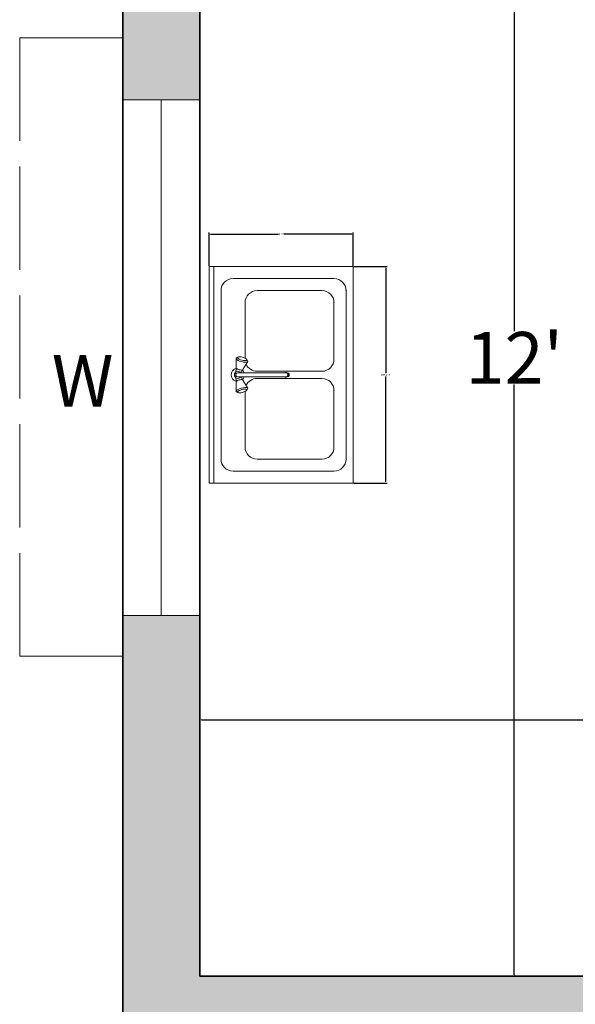
# Model space of a CAD drawing. Units: inches. Extents: x -5 to 482, y -460 to 66.
# Tile 17 of 31: x 21 to 86, y -143 to -29. Entities that reach past the tile are written whole.
import ezdxf

# ---------------------------------------------------------------- set-up
doc = ezdxf.new("R2010")
doc.units = ezdxf.units.IN
doc.header["$MEASUREMENT"] = 0
doc.linetypes.add('ACAD_ISO02W100', pattern=[15, 12, -3])
for name, color, linetype, lineweight in [('A-ANNO-DIMS', 2, 'Continuous', 18), ('A-ANNO-TEXT', 7, 'Continuous', 18), ('A-FLOR-FIXT', 9, 'Continuous', 18), ('A-GLAZ', 4, 'Continuous', 18), ('A-GLAZ-OVHD', 4, 'ACAD_ISO02W100', 13), ('A-WALL', 7, 'Continuous', 35), ('A-WALL-PATT', 152, 'Continuous', 13)]:
    doc.layers.add(name, color=color, linetype=linetype, lineweight=lineweight)
doc.styles.get("Standard").update_dxf_attribs({"font": 'arial.ttf'})
doc.dimstyles.get("Standard").update_dxf_attribs({"dimtxt": 0.18, "dimasz": 0.18, "dimexe": 0.18, "dimexo": 0.0625, "dimgap": 0.09, "dimtad": 0, "dimtih": 1, "dimtoh": 1, "dimdec": 0, "dimzin": 0, "dimdsep": 46, "dimlunit": 3, "dimtxsty": 'Standard', "dimcen": 0.09, "dimadec": 0, "dimazin": 0, "dimtfac": 1, "dimtdec": 0, "dimtofl": 0, "dimtmove": 0, "dimatfit": 3, "dimfxl": 1, "dimtolj": 1, "dimtzin": 0, "dimarcsym": 0})

# ---------------------------------------------------------------- blocks, each defined once
blk = doc.blocks.new('М07 600х900')
for p, q in [((0, 600), (-900, 600)), ((-900, 0), (-900, 600)), ((-900, 0), (-900, 600)), ((0, 580), (-900, 580)), ((0, 0), (0, 600)), ((0, 0), (0, 600)), ((-800, 550), (-100, 550)), ((-850, 80), (-850, 500)), ((-476.6, 488.7), (-472.7, 496.5)), ((-472.7, 496.5), (-466.5, 502.7)), ((-466.5, 502.7), (-458.7, 506.6)), ((-462.1, 488.8), (-454.6, 494.3)), ((-458.7, 506.6), (-450, 508)), ((-454.6, 494.3), (-445.4, 494.3)), ((-450, 508), (-441.3, 506.6)), ((-445.4, 494.3), (-437.9, 488.8)), ((-441.3, 506.6), (-433.5, 502.7)), ((-433.5, 502.7), (-427.3, 496.5)), ((-427.3, 496.5), (-423.4, 488.7)), ((-50, 500), (-50, 80)), ((-524.9, 472.1), (-524.8, 476.7)), ((-524.3, 466.5), (-524.9, 472.1)), ((-524.8, 476.7), (-523.8, 479.9)), ((-523, 460.4), (-524.3, 466.5)), ((-520.9, 485.6), (-523.8, 479.9)), ((-523.8, 479.9), (-522.2, 481.3)), ((-521.1, 454.5), (-523, 460.4)), ((-522.2, 481.3), (-520.1, 480.9)), ((-518.8, 449.4), (-521.1, 454.5)), ((-520.9, 485.6), (-518.9, 487.4)), ((-520.1, 480.9), (-517.7, 478.6)), ((-479.6, 487.6), (-518.9, 487.4)), ((-518.9, 487.4), (-516.3, 486.8)), ((-517.7, 478.6), (-515.3, 474.7)), ((-516.3, 486.8), (-513.3, 484)), ((-515.3, 474.7), (-513, 469.5)), ((-513.3, 484), (-510.2, 479.1)), ((-513, 469.5), (-511.1, 463.6)), ((-511.1, 463.6), (-509.8, 457.6)), ((-510.2, 479.1), (-507.4, 472.6)), ((-509.8, 457.6), (-509.2, 452)), ((-509.2, 452), (-509.4, 447.3)), ((-507.4, 472.6), (-505, 465.3)), ((-471.8, 458.6), (-506, 439.1)), ((-505, 465.3), (-503.4, 457.7)), ((-503.4, 457.7), (-502.6, 450.7)), ((-502.6, 450.7), (-502.8, 444.9)), ((-479.6, 487.6), (-478, 487.3)), ((-478, 487.3), (-476.2, 485.5)), ((-477, 486.3), (-476.6, 488.7)), ((-461.4, 489.4), (-476.2, 485.4)), ((-476.2, 485.5), (-474.4, 482.6)), ((-474.4, 482.6), (-472.7, 478.7)), ((-472.7, 478.7), (-471.2, 474.3)), ((-470.6, 459.7), (-471.8, 458.6)), ((-471.2, 474.3), (-470.3, 469.8)), ((-469.9, 462.1), (-470.6, 459.7)), ((-470.3, 469.8), (-469.8, 465.6)), ((-466.5, 457.3), (-470.2, 461.1)), ((-469.8, 465.6), (-469.9, 462.1)), ((-458.5, 465.3), (-469.9, 462.2)), ((-458.7, 453.4), (-466.5, 457.3)), ((-465, 480), (-462.1, 488.8)), ((-462.1, 471.2), (-465, 480)), ((-458.5, 468.5), (-462.1, 471.2)), ((-458.5, 453.3), (-458.7, 453.4)), ((-458.5, 480), (-456.9, 485)), ((-458.5, 480), (-458.5, 279.9)), ((-456.9, 485), (-452.6, 488.1)), ((-452.6, 488.1), (-447.4, 488.1)), ((-447.4, 488.1), (-443.1, 485)), ((-443.1, 485), (-441.5, 480)), ((-441.5, 480), (-441.5, 279.9)), ((-437.9, 471.2), (-441.5, 468.5)), ((-441.5, 465.3), (-430.1, 462.2)), ((-441.3, 453.4), (-441.5, 453.3)), ((-433.5, 457.3), (-441.3, 453.4)), ((-438.6, 489.4), (-423.8, 485.4)), ((-437.9, 488.8), (-435, 480)), ((-435, 480), (-437.9, 471.2)), ((-429.8, 461.1), (-433.5, 457.3)), ((-430.2, 465.6), (-429.7, 469.8)), ((-430.1, 462.1), (-430.2, 465.6)), ((-429.4, 459.7), (-430.1, 462.1)), ((-429.7, 469.8), (-428.8, 474.3)), ((-428.2, 458.6), (-429.4, 459.7)), ((-428.8, 474.3), (-427.3, 478.7)), ((-428.2, 458.6), (-394, 439.1)), ((-427.3, 478.7), (-425.6, 482.6)), ((-425.6, 482.6), (-423.8, 485.5)), ((-423.8, 485.5), (-422, 487.3)), ((-423.4, 488.7), (-423, 486.3)), ((-422, 487.3), (-420.4, 487.6)), ((-420.4, 487.6), (-381.1, 487.4)), ((-397.4, 450.7), (-396.6, 457.7)), ((-397.2, 444.9), (-397.4, 450.7)), ((-396.6, 457.7), (-395, 465.3)), ((-395, 465.3), (-392.6, 472.6)), ((-392.6, 472.6), (-389.8, 479.1)), ((-390.8, 452), (-390.2, 457.6)), ((-390.6, 447.3), (-390.8, 452)), ((-390.2, 457.6), (-388.9, 463.6)), ((-389.8, 479.1), (-386.7, 484)), ((-388.9, 463.6), (-387, 469.5)), ((-387, 469.5), (-384.7, 474.7)), ((-386.7, 484), (-383.7, 486.8)), ((-384.7, 474.7), (-382.3, 478.6)), ((-383.7, 486.8), (-381.1, 487.4)), ((-382.3, 478.6), (-379.9, 480.9)), ((-378.9, 454.5), (-381.2, 449.4)), ((-381.1, 487.4), (-379.1, 485.6)), ((-379.9, 480.9), (-377.8, 481.3)), ((-379.1, 485.6), (-376.2, 479.9)), ((-377, 460.4), (-378.9, 454.5)), ((-377.8, 481.3), (-376.2, 479.9)), ((-375.7, 466.5), (-377, 460.4)), ((-376.2, 479.9), (-375.2, 476.7)), ((-375.1, 472.1), (-375.7, 466.5)), ((-375.2, 476.7), (-375.1, 472.1)), ((-750, 450), (-519.1, 450)), ((-516.4, 445.5), (-518.8, 449.4)), ((-514, 443.2), (-516.4, 445.5)), ((-508.6, 439.7), (-514, 443.2)), ((-511.9, 442.7), (-514, 443.2)), ((-510.3, 444.2), (-511.9, 442.7)), ((-509.4, 447.3), (-510.3, 444.2)), ((-506, 439.1), (-508.6, 439.7)), ((-504, 440.9), (-506, 439.1)), ((-502.8, 444.9), (-504, 440.9)), ((-396, 440.9), (-397.2, 444.9)), ((-394, 439.1), (-396, 440.9)), ((-391.4, 439.7), (-394, 439.1)), ((-391.4, 439.7), (-386, 443.2)), ((-389.7, 444.2), (-390.6, 447.3)), ((-388.1, 442.7), (-389.7, 444.2)), ((-386, 443.2), (-388.1, 442.7)), ((-383.6, 445.5), (-386, 443.2)), ((-381.2, 449.4), (-383.6, 445.5)), ((-380.9, 450), (-150, 450)), ((-800, 130), (-800, 400)), ((-465, 400), (-465, 130)), ((-435, 130), (-435, 400)), ((-100, 400), (-100, 130)), ((-458.5, 285.6), (-460.5, 279.9)), ((-460.5, 279.9), (-458.5, 274.2)), ((-458.5, 279.9), (-456.9, 275.3)), ((-458.5, 274.2), (-456.9, 269.8)), ((-458.5, 274.2), (-453.2, 270.6)), ((-456.9, 275.3), (-452.6, 272.4)), ((-456.9, 269.8), (-452.6, 266.9)), ((-453.2, 270.6), (-446.8, 270.6)), ((-452.6, 272.4), (-447.4, 272.4)), ((-452.6, 266.9), (-447.4, 266.9)), ((-447.4, 272.4), (-443.1, 275.3)), ((-447.4, 266.9), (-443.1, 269.8)), ((-446.8, 270.6), (-441.5, 274.2)), ((-443.1, 275.3), (-441.5, 279.9)), ((-441.5, 274.2), (-443.1, 269.8)), ((-439.5, 279.9), (-441.5, 285.6)), ((-441.5, 274.2), (-439.5, 279.9)), ((-515, 80), (-750, 80)), ((-150, 80), (-385, 80)), ((0, 0), (-900, 0)), ((-100, 30), (-800, 30))]:
    blk.add_line(p, q)
for centre, start, end in [((-800, 500), 90, 180), ((-100, 500), 0, 90), ((-750, 400), 90, 180), ((-515, 400), 0, 65.8874), ((-385, 400), 114.1126, 180), ((-150, 400), 0, 90), ((-750, 130), 180, 270), ((-515, 130), 270, 0), ((-385, 130), 180, 270), ((-150, 130), 270, 0), ((-800, 80), 180, 270), ((-100, 80), 270, 0)]:
    blk.add_arc(centre, 50, start, end)
for p in [(-515, 80), (-150, 80), (-100, 30)]:
    blk.add_point(p)
blk = doc.blocks.new('*D5')
at = {"layer": 'A-ANNO-DIMS', "color": 0, "lineweight": -2, "transparency": 16777216}
for p, q in [((41.88, -113.79), (41.88, -109.8)), ((42.06, -109.98), (93.03, -109.98)), ((149.7, -109.98), (98.73, -109.98)), ((149.88, -113.79), (149.88, -109.8))]:
    blk.add_line(p, q, dxfattribs=at)
at = {"layer": 'A-ANNO-DIMS', "color": 0, "transparency": 16777216}
for points in [[(42.06, -109.95), (42.06, -110.01), (41.88, -109.98)], [(149.7, -109.95), (149.7, -110.01), (149.88, -109.98)]]:
    blk.add_solid(points, dxfattribs=at)
at = {"layer": 'Defpoints', "color": 0, "transparency": 16777216}
for p in [(41.88, -109.98), (41.88, -113.85), (149.88, -113.85)]:
    blk.add_point(p, dxfattribs=at)
at = {"layer": 'A-ANNO-DIMS', "color": 0, "transparency": 16777216, "insert": (95.88, -109.98), "char_height": 6, "attachment_point": 5}
blk.add_mtext("\\A1;9'", dxfattribs=at)
blk = doc.blocks.new('*D6')
at = {"layer": 'A-ANNO-DIMS', "color": 0, "lineweight": -2, "transparency": 16777216}
for p, q in [((78.66, 4.15), (78.33, 4.15)), ((78.51, 3.97), (78.51, -64.75)), ((78.51, -139.67), (78.51, -70.95)), ((78.66, -139.85), (78.33, -139.85))]:
    blk.add_line(p, q, dxfattribs=at)
at = {"layer": 'A-ANNO-DIMS', "color": 0, "transparency": 16777216}
for points in [[(78.48, 3.97), (78.54, 3.97), (78.51, 4.15)], [(78.48, -139.67), (78.54, -139.67), (78.51, -139.85)]]:
    blk.add_solid(points, dxfattribs=at)
at = {"layer": 'Defpoints', "color": 0, "transparency": 16777216}
for p in [(78.72, 4.15), (78.51, -139.85), (78.72, -139.85)]:
    blk.add_point(p, dxfattribs=at)
at = {"layer": 'A-ANNO-DIMS', "color": 0, "transparency": 16777216, "insert": (78.51, -67.85), "char_height": 6, "attachment_point": 5}
blk.add_mtext("\\A1;12'", dxfattribs=at)
blk = doc.blocks.new('WIN-GLAZ-60IN')
for p, q in [((0, 9), (60, 9)), ((0, 4.5), (60, 4.5)), ((60, 0), (0, 0))]:
    blk.add_line(p, q)
blk = doc.blocks.new('WIN-SHADE-72IN')
for p, q in [((0, 12), (72, 12)), ((0, 12), (0, 0)), ((72, 12), (72, 0))]:
    blk.add_line(p, q)
blk = doc.blocks.new('*D67')
at = {"layer": 'A-ANNO-DIMS', "color": 0, "lineweight": -2, "transparency": 16777216}
for p, q in [((59.8, -57.24), (63.7, -57.24)), ((63.52, -57.42), (63.52, -69.66)), ((63.52, -82.26), (63.52, -70.02)), ((59.8, -82.44), (63.7, -82.44))]:
    blk.add_line(p, q, dxfattribs=at)
at = {"layer": 'A-ANNO-DIMS', "color": 0, "transparency": 16777216}
for points in [[(63.49, -57.42), (63.55, -57.42), (63.52, -57.24)], [(63.49, -82.26), (63.55, -82.26), (63.52, -82.44)]]:
    blk.add_solid(points, dxfattribs=at)
at = {"layer": 'Defpoints', "color": 0, "transparency": 16777216}
for p in [(59.74, -57.24), (63.52, -57.24), (59.74, -82.44)]:
    blk.add_point(p, dxfattribs=at)
at = {"layer": 'A-ANNO-DIMS', "color": 0, "transparency": 16777216, "insert": (63.52, -69.84), "char_height": 0.18, "attachment_point": 5}
blk.add_mtext('\\A1;SINK 2\'-1"', dxfattribs=at)
blk = doc.blocks.new('*D68')
at = {"layer": 'A-ANNO-DIMS', "color": 0, "lineweight": -2, "transparency": 16777216}
for p, q in [((42.94, -57.17), (42.94, -53.28)), ((43.12, -53.46), (51.02, -53.46)), ((59.56, -53.46), (51.66, -53.46)), ((59.74, -57.17), (59.74, -53.28))]:
    blk.add_line(p, q, dxfattribs=at)
at = {"layer": 'A-ANNO-DIMS', "color": 0, "transparency": 16777216}
for points in [[(43.12, -53.43), (43.12, -53.49), (42.94, -53.46)], [(59.56, -53.43), (59.56, -53.49), (59.74, -53.46)]]:
    blk.add_solid(points, dxfattribs=at)
at = {"layer": 'Defpoints', "color": 0, "transparency": 16777216}
for p in [(42.94, -53.46), (42.94, -57.24), (59.74, -57.24)]:
    blk.add_point(p, dxfattribs=at)
at = {"layer": 'A-ANNO-DIMS', "color": 0, "transparency": 16777216, "insert": (51.34, -53.46), "char_height": 0.18, "attachment_point": 5}
blk.add_mtext('\\A1;1\'-5"', dxfattribs=at)

msp = doc.modelspace()

# ---------------------------------------------------------------- hatches: boundary and pattern name
at = {"layer": 'A-WALL-PATT'}
h = msp.add_hatch(color=256, dxfattribs=at)
h.dxf.hatch_style = 1
h.paths.add_polyline_path([(149.38, -412.85), (144.38, -412.85), (144.38, -283.85), (144.38, -279.35), (133.88, -279.35), (133.88, -283.85), (139.88, -283.85), (139.88, -412.85), (133.51, -412.85), (133.51, -413.92), (102.65, -413.92), (102.65, -421.02), (133.51, -421.02), (133.51, -421.85), (149.38, -421.85)])
h.paths.add_polyline_path([(226.05, -412.85), (218.88, -412.85), (218.88, -350.85), (262.88, -350.85), (262.88, -386.85), (267.38, -386.85), (267.38, -283.85), (270.38, -283.85), (270.38, -279.35), (244.88, -279.35), (244.88, -283.85), (262.88, -283.85), (262.88, -346.35), (218.88, -346.35), (218.88, -283.85), (220.88, -283.85), (220.88, -279.35), (214.38, -279.35), (214.38, -283.85), (214.38, -412.85), (209.38, -412.85), (209.38, -421.85), (226.05, -421.85)])
h.paths.add_polyline_path([(315.81, -412.85), (250.05, -412.85), (250.05, -421.85), (315.81, -421.85)])
h.paths.add_polyline_path([(430.38, -378.35), (421.38, -378.35), (421.38, -412.85), (375.81, -412.85), (375.81, -421.85), (430.38, -421.85)])
h.paths.add_polyline_path([(78.69, -413.92), (47.68, -413.92), (47.68, -412.85), (41.88, -412.85), (41.88, -283.85), (109.88, -283.85), (109.88, -279.35), (41.88, -279.35), (41.88, -241.85), (32.88, -241.85), (32.88, -421.85), (47.68, -421.85), (47.68, -421.02), (78.69, -421.02)])
h.paths.add_polyline_path([(41.88, -144.35), (154.38, -144.35), (154.38, -137.85), (149.88, -137.85), (149.88, -139.85), (41.88, -139.85), (41.88, -97.85), (32.88, -97.85), (32.88, -181.85), (41.88, -181.85)])
h.paths.add_polyline_path([(430.38, -241.85), (421.38, -241.85), (421.38, -279.35), (309.38, -279.35), (309.38, -170.35), (304.88, -170.35), (304.88, -279.35), (294.38, -279.35), (294.38, -283.85), (421.38, -283.85), (421.38, -318.35), (430.38, -318.35)])
h.paths.add_polyline_path([(430.38, -119.85), (421.38, -119.85), (421.38, -139.85), (419.38, -139.85), (419.38, -144.35), (421.38, -144.35), (421.38, -181.85), (430.38, -181.85)])
h.paths.add_polyline_path([(395.38, -139.85), (377.38, -139.85), (377.38, -75.85), (421.38, -75.85), (421.38, -95.85), (430.38, -95.85), (430.38, -45.6), (421.38, -45.6), (421.38, -71.35), (377.38, -71.35), (377.38, -22.85), (372.88, -22.85), (372.88, -139.85), (242.88, -139.85), (242.88, -137.85), (238.38, -137.85), (238.38, -144.35), (304.88, -144.35), (304.88, -146.35), (309.38, -146.35), (309.38, -144.35), (395.38, -144.35)])
h.paths.add_polyline_path([(65.88, 13.15), (32.88, 13.15), (32.88, -37.85), (41.88, -37.85), (41.88, 4.15), (65.88, 4.15)])
h.paths.add_polyline_path([(166.38, 13.15), (125.88, 13.15), (125.88, 4.15), (149.88, 4.15), (149.88, -113.85), (154.38, -113.85), (154.38, 4.15), (166.38, 4.15)])
h.paths.add_polyline_path([(277.88, 13.15), (226.38, 13.15), (226.38, 4.15), (238.38, 4.15), (238.38, -113.85), (242.88, -113.85), (242.88, 4.15), (277.88, 4.15)])
h.paths.add_polyline_path([(430.38, 13.15), (337.88, 13.15), (337.88, 4.15), (372.88, 4.15), (372.88, 1.15), (377.38, 1.15), (377.38, 4.15), (421.38, 4.15), (421.38, -21.6), (430.38, -21.6)])

# ---------------------------------------------------------------- linework, layer by layer
at = {"layer": 'A-GLAZ'}
for p, q in [((41.88, -37.85), (32.88, -37.85)), ((32.88, -97.85), (41.88, -97.85))]:
    msp.add_line(p, q, dxfattribs=at)
at = {"layer": 'A-WALL'}
for p, q in [((32.88, 13.15), (32.88, -421.85)), ((41.88, 4.15), (41.88, -139.85)), ((41.88, -139.85), (149.88, -139.85))]:
    msp.add_line(p, q, dxfattribs=at)

# ---------------------------------------------------------------- block references
at = {"layer": 'A-FLOR-FIXT', "xscale": 0.0280055379010044, "yscale": 0.0280055379010044, "zscale": 0.0280055379010044, "rotation": 90}
msp.add_blockref('М07 600х900', (59.74, -57.24), dxfattribs=at)
at = {"layer": 'A-GLAZ', "rotation": 90.00000000000003}
msp.add_blockref('WIN-GLAZ-60IN', (41.88, -97.85), dxfattribs=at)
at = {"layer": 'A-GLAZ-OVHD', "rotation": 90}
msp.add_blockref('WIN-SHADE-72IN', (32.88, -102.6), dxfattribs=at)

# ---------------------------------------------------------------- texts
at = {"layer": 'A-ANNO-TEXT', "insert": (24.62, -67.54), "char_height": 6, "attachment_point": 1}
msp.add_mtext('W', dxfattribs=at)

# ---------------------------------------------------------------- dimensions: what is measured, and where the dimension line sits
at = {"layer": 'A-ANNO-DIMS'}
for base, p1, p2, angle, override, picture, middle in [((78.51, -139.85), (78.72, 4.15), (78.72, -139.85), 90, {"dimtxt": 6, "dimclrd": 0, "dimclre": 0, "dimclrt": 0}, '*D6', (78.51, -67.85)), ((42.94, -53.46), (59.74, -57.24), (42.94, -57.24), 180, {"dimdec": 1, "dimlfac": 1, "dimrnd": 0, "dimzin": 1, "dimdsep": 46, "dimlunit": 4, "dimfrac": 2}, '*D68', (51.34, -53.46))]:
    dim = msp.add_linear_dim(base=base, p1=p1, p2=p2, angle=angle, dimstyle='Standard', override=override, dxfattribs=at)
    dim.commit()
    dim.dimension.update_dxf_attribs({"geometry": picture, "text_midpoint": middle})
dim = msp.add_linear_dim(base=(63.52, -57.24), p1=(59.74, -82.44), p2=(59.74, -57.24), angle=90, text='SINK <>', dimstyle='Standard', override={"dimdec": 1, "dimlfac": 1, "dimrnd": 0, "dimzin": 1, "dimdsep": 46, "dimlunit": 4, "dimfrac": 2}, dxfattribs=at)
dim.commit()
dim.dimension.update_dxf_attribs({"geometry": '*D67', "text_midpoint": (63.52, -69.84)})
dim = msp.add_linear_dim(base=(41.88, -109.98), p1=(149.88, -113.85), p2=(41.88, -113.85), dimstyle='Standard', override={"dimtxt": 6, "dimclrd": 0, "dimclre": 0, "dimclrt": 0}, dxfattribs=at)
dim.commit()
dim.dimension.update_dxf_attribs({"geometry": '*D5', "text_midpoint": (95.88, -109.98)})

doc.saveas('drawing.dxf')
